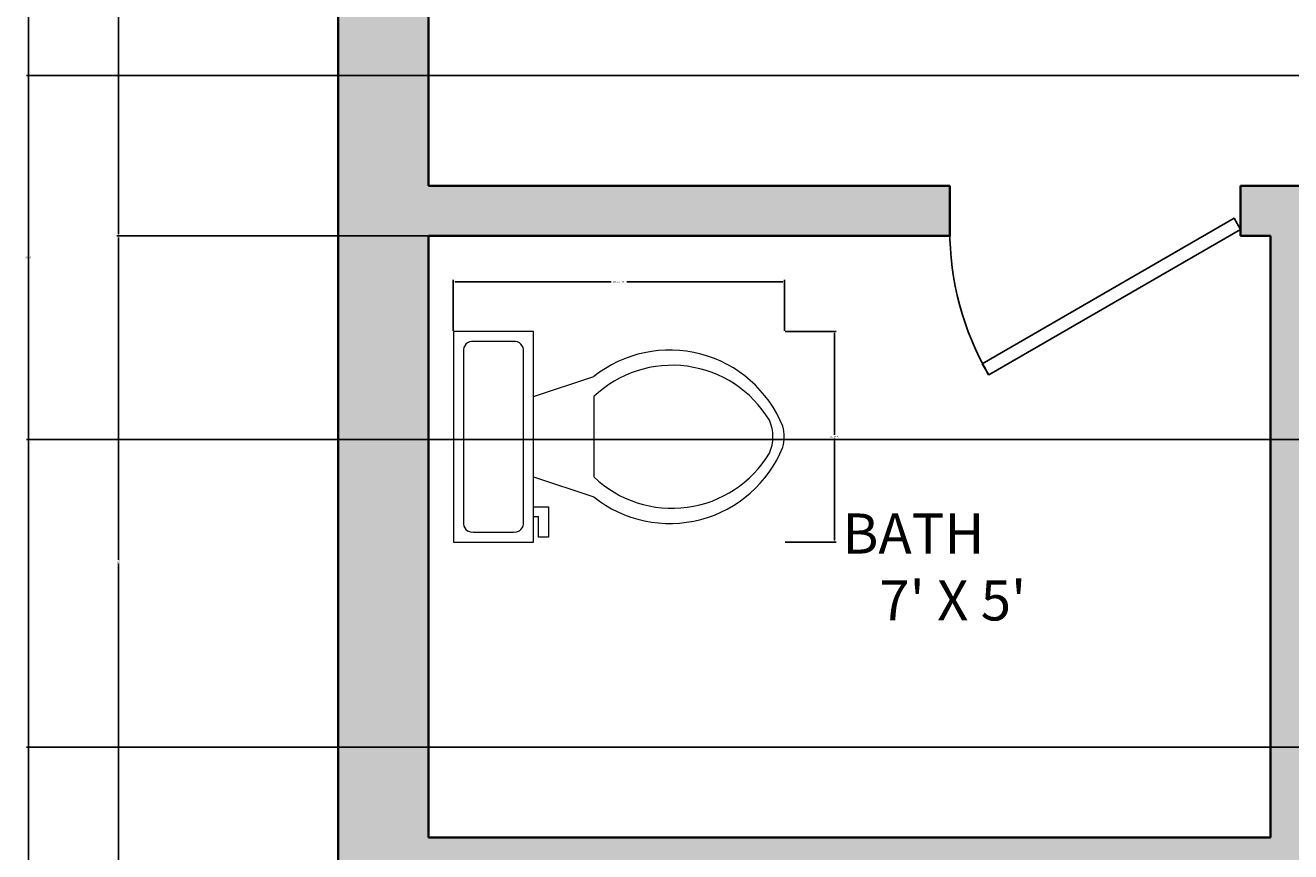
# Model space of a CAD drawing. Units: inches. Extents: x -30 to 437, y -29 to 647.
# Tile 3 of 15: x -30 to 97, y 172 to 255. Entities that reach past the tile are written whole.
import ezdxf

# ---------------------------------------------------------------- set-up
doc = ezdxf.new("R2010")
doc.units = ezdxf.units.IN
doc.header["$MEASUREMENT"] = 0
for name, color, linetype, lineweight in [('A-ANNO-DIMS', 2, 'Continuous', 18), ('A-AREA-IDEN', 7, 'Continuous', 18), ('A-WALL', 7, 'Continuous', 35), ('bathroom', 90, 'Continuous', 18), ('doors', 40, 'Continuous', 25)]:
    doc.layers.add(name, color=color, linetype=linetype, lineweight=lineweight)
doc.layers.add('A-WALL-PATT', color=251, linetype='Continuous', lineweight=13, true_color=0x636466)
doc.styles.get("Standard").update_dxf_attribs({"font": 'arial.ttf'})
doc.dimstyles.get("Standard").update_dxf_attribs({"dimtxt": 0.18, "dimasz": 0.18, "dimexe": 0.18, "dimexo": 0.0625, "dimgap": 0.09, "dimtad": 0, "dimtih": 1, "dimtoh": 1, "dimdec": 4, "dimzin": 0, "dimdsep": 46, "dimtxsty": 'Standard', "dimcen": 0.09, "dimadec": 0, "dimazin": 0, "dimtfac": 1, "dimtdec": 4, "dimtofl": 0, "dimtmove": 0, "dimatfit": 3, "dimfxl": 1, "dimtolj": 1, "dimtzin": 0, "dimarcsym": 0})

# ---------------------------------------------------------------- blocks, each defined once
blk = doc.blocks.new('Toilet - top')
for p, q in [((9.5, -6), (9.5, -2)), ((-10, -8.5), (-8, -8.5)), ((-10, -9.5), (-10, -8.5)), ((-8, -8.5), (-8, -8)), ((-7, -8), (-7, -9.5)), ((-4, -8), (-6, -14)), ((4, -8), (6, -14)), ((-7, -9.5), (-10, -9.5)), ((4, -14), (-4, -14))]:
    blk.add_line(p, q)
blk.add_lwpolyline([(10.5, -8), (10.5, 0), (-10.5, 0), (-10.5, -8)], close=True)
for points in [[(8.5, -1), (-8.5, -1)], [(-9.5, -2), (-9.5, -6)], [(-8.5, -7), (8.5, -7)]]:
    blk.add_lwpolyline(points)
for centre, radius, start, end in [((-8.62, -1.88), 0.884, 81.8699, 188.1301), ((8.62, -1.88), 0.884, 351.8699, 98.1301), ((-8.62, -6.12), 0.884, 171.8699, 278.1301), ((8.62, -6.12), 0.884, 261.8699, 8.1301), ((3.52, -21.58), 12.17, 141.4691, 247.9714), ((4.2, -21.82), 11.33, 136.3677, 238.9468), ((-3.52, -21.58), 12.17, 292.0284, 38.5307), ((-4.2, -21.82), 11.33, 301.053, 43.6321), ((0, -27.88), 4, 245.7318, 294.2682), ((0, -29), 4, 254.8605, 285.1395)]:
    blk.add_arc(centre, radius, start, end)
blk = doc.blocks.new('*U6')
for p, q in [((0, 0), (0, -6)), ((40, 0), (40, -6))]:
    blk.add_line(p, q)
blk.add_lwpolyline([(0, 0), (34.64, 20), (35.52, 18.48), (0.87, -1.52)], close=True)
blk.add_arc((0, 0), 40, 0, 30)
blk = doc.blocks.new('*D13')
at = {"layer": 'A-ANNO-DIMS', "color": 0, "lineweight": -2, "transparency": 16777216}
for p, q in [((13.16, 224.07), (13.16, 229.15)), ((13.34, 228.97), (28.91, 228.97)), ((46.03, 228.97), (30.46, 228.97)), ((46.21, 224.07), (46.21, 229.15))]:
    blk.add_line(p, q, dxfattribs=at)
at = {"layer": 'A-ANNO-DIMS', "color": 0, "transparency": 16777216}
for points in [[(13.34, 229), (13.34, 228.94), (13.16, 228.97)], [(46.03, 229), (46.03, 228.94), (46.21, 228.97)]]:
    blk.add_solid(points, dxfattribs=at)
at = {"layer": 'Defpoints', "color": 0, "transparency": 16777216}
for p in [(13.16, 228.97), (13.16, 224.01), (46.21, 224.01)]:
    blk.add_point(p, dxfattribs=at)
at = {"layer": 'A-ANNO-DIMS', "color": 0, "transparency": 16777216, "insert": (29.69, 228.97), "char_height": 0.18, "attachment_point": 5}
blk.add_mtext('\\A1;WC 33 TYP.', dxfattribs=at)
blk = doc.blocks.new('*D14')
at = {"layer": 'A-ANNO-DIMS', "color": 0, "lineweight": -2, "transparency": 16777216}
for p, q in [((46.27, 224.01), (51.35, 224.01)), ((51.17, 223.83), (51.17, 213.69)), ((51.17, 203.19), (51.17, 213.33)), ((46.27, 203.01), (51.35, 203.01))]:
    blk.add_line(p, q, dxfattribs=at)
at = {"layer": 'A-ANNO-DIMS', "color": 0, "transparency": 16777216}
for points in [[(51.14, 223.83), (51.2, 223.83), (51.17, 224.01)], [(51.14, 203.19), (51.2, 203.19), (51.17, 203.01)]]:
    blk.add_solid(points, dxfattribs=at)
at = {"layer": 'Defpoints', "color": 0, "transparency": 16777216}
for p in [(46.21, 224.01), (51.17, 224.01), (46.21, 203.01)]:
    blk.add_point(p, dxfattribs=at)
at = {"layer": 'A-ANNO-DIMS', "color": 0, "transparency": 16777216, "insert": (51.17, 213.51), "char_height": 0.18, "attachment_point": 5}
blk.add_mtext('\\A1;21 TYP.', dxfattribs=at)
blk = doc.blocks.new('*D26')
at = {"layer": 'A-ANNO-DIMS', "color": 0, "lineweight": -2, "transparency": 16777216}
for p, q in [((1.61, 615.55), (-29.41, 615.55)), ((-29.23, 615.37), (-29.23, 308.98)), ((-29.23, 2.23), (-29.23, 308.62)), ((1.61, 2.05), (-29.41, 2.05))]:
    blk.add_line(p, q, dxfattribs=at)
at = {"layer": 'A-ANNO-DIMS', "color": 0, "transparency": 16777216}
for points in [[(-29.26, 615.37), (-29.2, 615.37), (-29.23, 615.55)], [(-29.26, 2.23), (-29.2, 2.23), (-29.23, 2.05)]]:
    blk.add_solid(points, dxfattribs=at)
at = {"layer": 'Defpoints', "color": 0, "transparency": 16777216}
for p in [(-29.23, 615.55), (1.67, 615.55), (1.67, 2.05)]:
    blk.add_point(p, dxfattribs=at)
at = {"layer": 'A-ANNO-DIMS', "color": 0, "transparency": 16777216, "insert": (-29.23, 308.8), "char_height": 0.18, "attachment_point": 5}
blk.add_mtext('\\A1;613.5', dxfattribs=at)
blk = doc.blocks.new('*D31')
at = {"layer": 'A-ANNO-DIMS', "color": 0, "lineweight": -2, "transparency": 16777216}
for p, q in [((10.61, 233.55), (-20.41, 233.55)), ((-20.23, 233.37), (-20.23, 201.23)), ((-20.23, 168.73), (-20.23, 200.87)), ((10.61, 168.55), (-20.41, 168.55))]:
    blk.add_line(p, q, dxfattribs=at)
at = {"layer": 'A-ANNO-DIMS', "color": 0, "transparency": 16777216}
for points in [[(-20.26, 233.37), (-20.2, 233.37), (-20.23, 233.55)], [(-20.26, 168.73), (-20.2, 168.73), (-20.23, 168.55)]]:
    blk.add_solid(points, dxfattribs=at)
at = {"layer": 'Defpoints', "color": 0, "transparency": 16777216}
for p in [(-20.23, 233.55), (10.67, 233.55), (10.67, 168.55)]:
    blk.add_point(p, dxfattribs=at)
at = {"layer": 'A-ANNO-DIMS', "color": 0, "transparency": 16777216, "insert": (-20.23, 201.05), "char_height": 0.18, "attachment_point": 5}
blk.add_mtext('\\A1;65', dxfattribs=at)
blk = doc.blocks.new('*D32')
at = {"layer": 'A-ANNO-DIMS', "color": 0, "lineweight": -2, "transparency": 16777216}
for p, q in [((10.61, 386.55), (-20.41, 386.55)), ((-20.23, 386.37), (-20.23, 310.23)), ((-20.23, 233.73), (-20.23, 309.87)), ((10.61, 233.55), (-20.41, 233.55))]:
    blk.add_line(p, q, dxfattribs=at)
at = {"layer": 'A-ANNO-DIMS', "color": 0, "transparency": 16777216}
for points in [[(-20.26, 386.37), (-20.2, 386.37), (-20.23, 386.55)], [(-20.26, 233.73), (-20.2, 233.73), (-20.23, 233.55)]]:
    blk.add_solid(points, dxfattribs=at)
at = {"layer": 'Defpoints', "color": 0, "transparency": 16777216}
for p in [(-20.23, 386.55), (10.67, 386.55), (10.67, 233.55)]:
    blk.add_point(p, dxfattribs=at)
at = {"layer": 'A-ANNO-DIMS', "color": 0, "transparency": 16777216, "insert": (-20.23, 310.05), "char_height": 0.18, "attachment_point": 5}
blk.add_mtext('\\A1;153', dxfattribs=at)
blk = doc.blocks.new('*D52')
at = {"layer": 'A-ANNO-DIMS', "color": 0, "lineweight": -2, "transparency": 16777216}
for p, q in [((367.61, 182.55), (-29.41, 182.55)), ((-29.23, 182.37), (-29.23, 168.23)), ((-29.23, 153.73), (-29.23, 167.87)), ((396.61, 153.55), (-29.41, 153.55))]:
    blk.add_line(p, q, dxfattribs=at)
at = {"layer": 'A-ANNO-DIMS', "color": 0, "transparency": 16777216}
for points in [[(-29.26, 182.37), (-29.2, 182.37), (-29.23, 182.55)], [(-29.26, 153.73), (-29.2, 153.73), (-29.23, 153.55)]]:
    blk.add_solid(points, dxfattribs=at)
at = {"layer": 'Defpoints', "color": 0, "transparency": 16777216}
for p in [(367.67, 182.55), (-29.23, 153.55), (396.67, 153.55)]:
    blk.add_point(p, dxfattribs=at)
at = {"layer": 'A-ANNO-DIMS', "color": 0, "transparency": 16777216, "insert": (-29.23, 168.05), "char_height": 0.18, "attachment_point": 5}
blk.add_mtext('\\A1;29', dxfattribs=at)
blk = doc.blocks.new('*D55')
at = {"layer": 'A-ANNO-DIMS', "color": 0, "lineweight": -2, "transparency": 16777216}
for p, q in [((367.61, 249.55), (-29.41, 249.55)), ((-29.23, 249.37), (-29.23, 231.57)), ((-29.23, 213.42), (-29.23, 231.21)), ((369.54, 213.24), (-29.41, 213.24))]:
    blk.add_line(p, q, dxfattribs=at)
at = {"layer": 'A-ANNO-DIMS', "color": 0, "transparency": 16777216}
for points in [[(-29.26, 249.37), (-29.2, 249.37), (-29.23, 249.55)], [(-29.26, 213.42), (-29.2, 213.42), (-29.23, 213.24)]]:
    blk.add_solid(points, dxfattribs=at)
at = {"layer": 'Defpoints', "color": 0, "transparency": 16777216}
for p in [(-29.23, 249.55), (367.67, 249.55), (369.61, 213.24)]:
    blk.add_point(p, dxfattribs=at)
at = {"layer": 'A-ANNO-DIMS', "color": 0, "transparency": 16777216, "insert": (-29.23, 231.39), "char_height": 0.18, "attachment_point": 5}
blk.add_mtext('\\A1;36.31', dxfattribs=at)

msp = doc.modelspace()

# ---------------------------------------------------------------- hatches: boundary and pattern name
at = {"layer": 'A-WALL-PATT'}
h = msp.add_hatch(color=256, dxfattribs=at)
h.dxf.hatch_style = 1
h.paths.add_polyline_path([(393.6054, 183.2352), (369.6054, 183.2352), (369.6054, 213.2352), (393.6054, 213.2352), (393.6054, 207.2352), (394.6054, 207.2352), (394.6054, 211.2352), (395.6054, 211.2352), (395.6054, 185.2352), (394.6054, 185.2352), (394.6054, 189.2352), (393.6054, 189.2352)], flags=0)
h.paths.add_polyline_path([(384.6054, 189.2352, -1), (390.6054, 189.2352, -1)], flags=0)
h.paths.add_polyline_path([(385.6054, 189.2352, -1), (389.6054, 189.2352, -1)], flags=0)
h.paths.add_polyline_path([(374.6054, 189.2352, -1), (382.6054, 189.2352, -1)], flags=0)
h.paths.add_polyline_path([(386.6054, 189.2352, -1), (388.6054, 189.2352, -1)], flags=0)
h.paths.add_polyline_path([(375.6054, 189.2352, -1), (381.6054, 189.2352, -1)], flags=0)
h.paths.add_polyline_path([(376.6054, 189.2352, -1), (380.6054, 189.2352, -1)], flags=0)
h.paths.add_polyline_path([(377.6054, 189.2352, -1), (379.6054, 189.2352, -1)], flags=0)
h.paths.add_polyline_path([(390.6054, 195.2352), (374.6054, 195.2352), (374.6054, 201.2352), (390.6054, 201.2352)], flags=0)
h.paths.add_polyline_path([(389.6054, 196.2352), (375.6054, 196.2352), (375.6054, 200.2352), (389.6054, 200.2352)], flags=0)
h.paths.add_polyline_path([(383.6054, 207.2352, -1), (391.6054, 207.2352, -1)], flags=0)
h.paths.add_polyline_path([(384.6054, 207.2352, -1), (390.6054, 207.2352, -1)], flags=0)
h.paths.add_polyline_path([(385.6054, 207.2352, -1), (389.6054, 207.2352, -1)], flags=0)
h.paths.add_polyline_path([(386.6054, 207.2352, -1), (388.6054, 207.2352, -1)], flags=0)
h.paths.add_polyline_path([(375.6054, 207.2352, -1), (381.6054, 207.2352, -1)], flags=0)
h.paths.add_polyline_path([(376.6054, 207.2352, -1), (380.6054, 207.2352, -1)], flags=0)
h.paths.add_polyline_path([(377.6054, 207.2352, -1), (379.6054, 207.2352, -1)], flags=0)
h.paths.add_polyline_path([(305.5437, 160.3663, -0.41421356), (304.0437, 158.8663), (271.0437, 158.8663, -0.41421356), (269.5437, 160.3663), (269.5437, 178.3663, -0.41421356), (271.0437, 179.8663), (304.0437, 179.8663, -0.41421356), (305.5437, 178.3663)], flags=0)
h.paths.add_polyline_path([(304.0437, 165.3663, -0.41421356), (303.0437, 164.3663), (289.2937, 164.3663, -0.41421356), (288.2937, 165.3663), (288.2937, 177.3663, -0.41421356), (289.2937, 178.3663), (303.0437, 178.3663, -0.41421356), (304.0437, 177.3663)], flags=0)
h.paths.add_polyline_path([(296.5437, 171.3663, -1), (295.5437, 171.3663, -1)], flags=0)
h.paths.add_polyline_path([(286.7937, 165.3663, -0.41421356), (285.7937, 164.3663), (272.0437, 164.3663, -0.41421356), (271.0437, 165.3663), (271.0437, 177.3663, -0.41421356), (272.0437, 178.3663), (285.7937, 178.3663, -0.41421356), (286.7937, 177.3663)], flags=0)
h.paths.add_polyline_path([(279.5437, 171.3663, -1), (278.5437, 171.3663, -1)], flags=0)
h.paths.add_polyline_path([(360.6737, 290.5474), (360.6737, 300.5474), (396.6737, 300.5474), (396.6737, 290.5474)], flags=0)
h.paths.add_polyline_path([(259.6737, 124.5474), (259.6737, 114.5474), (171.6737, 114.5474), (171.6737, 124.5474)], flags=0)
h.paths.add_polyline_path([(288.0737, 215.3705), (286.7097, 214.583), (268.7097, 245.7599), (270.0737, 246.5474)], flags=0)
h.paths.add_polyline_path([(259.6737, 168.5474), (256.6737, 168.5474), (256.6737, 173.5474), (256.6737, 179.0224), (255.8753, 177.6395), (224.2956, 195.872, 0.12053744), (220.1737, 179.0224, 0.12053744), (216.0518, 195.872), (184.4721, 177.6395), (183.6737, 179.0224), (215.2836, 197.2724), (216.0821, 195.8895), (216.0518, 195.872, -0.12053744), (220.1737, 179.0224, -0.12053744), (224.2956, 195.872), (224.2653, 195.8895), (225.0638, 197.2724), (256.6737, 179.0224), (256.6737, 173.5474), (259.6737, 173.5474)], flags=0)
h.paths.add_polyline_path([(386.7943, 325.4601), (372.6871, 325.4601), (372.6871, 339.5673), (386.7943, 339.5673)], flags=0)
h.paths.add_polyline_path([(359.5875, 343.7429), (357.7905, 343.7429), (357.7905, 327.9179), (359.3933, 327.9179, 0.41420885), (361.5302, 330.0549), (361.5302, 341.8434, 0.41436161)], flags=0)
h.paths.add_polyline_path([(341.7887, 323.1235, -0.11921667), (340.7839, 323.1235)], flags=0)
h.paths.add_polyline_path([(379.6332, 328.8632), (379.6332, 332.2699), (376.0992, 332.2699, 0.39427733)], flags=0)
h.paths.add_polyline_path([(375.5299, 332.459, -1), (383.8511, 332.459, -1)], flags=0)
h.paths.add_polyline_path([(388.9363, 344.7425), (372.5309, 344.7425, -0.41421356), (370.394, 346.8794), (370.394, 347.5594, -0.39085173), (372.3472, 349.7005, -0.43951011), (370.394, 351.4933), (370.394, 365.1894, -0.40305452), (372.2191, 367.1298, -0.41839453), (370.394, 368.9291), (370.394, 382.6251, -0.40885826), (372.2519, 384.5722, -0.42377324), (370.394, 386.3707), (370.394, 400.0667, -0.38660687), (372.1327, 402.0094), (372.531, 402.0094, -0.41421834), (370.394, 404.1464), (370.394, 404.7778, -0.41420891), (372.5309, 406.9147), (388.9363, 406.9147, -0.41421821), (391.0733, 404.7778), (391.0733, 346.8794, -0.41421356)], flags=0)
edge = h.paths.add_edge_path(flags=0)
edge.add_spline(control_points=[(349.3585, 363.204), (349.0859, 363.204), (348.8133, 363.2227), (348.2712, 363.2973), (348.0016, 363.3531), (347.3533, 363.5328), (346.9776, 363.6755), (346.2445, 364.0308), (345.887, 364.2432), (345.1953, 364.7329), (344.8611, 365.0101), (344.2197, 365.6237), (343.9125, 365.9603), (343.211, 366.8336), (342.8313, 367.3965), (342.1401, 368.6117), (341.8286, 369.2641), (341.2807, 370.64), (341.0443, 371.3636), (340.6522, 372.8619), (340.4964, 373.6367), (340.2695, 375.2158), (340.1983, 376.0203), (340.142, 377.6365), (340.157, 378.4483), (340.2729, 380.0567), (340.3738, 380.8533), (340.6589, 382.4093), (340.8432, 383.1686), (341.2906, 384.629), (341.5538, 385.3301), (342.1531, 386.6544), (342.4891, 387.2776), (343.2266, 388.4288), (343.6281, 388.9567), (344.4879, 389.9012), (344.9463, 390.3178), (345.7981, 390.9428), (346.182, 391.1771), (346.9712, 391.5648), (347.3766, 391.7182), (348.2004, 391.9387), (348.6189, 392.0058), (349.4588, 392.0508), (349.8801, 392.0288), (350.7146, 391.8966), (351.1278, 391.7865), (351.9366, 391.4822), (352.3323, 391.2882), (353.0989, 390.8223), (353.4699, 390.5504), (354.1819, 389.9355), (354.5229, 389.5924), (355.1706, 388.8418), (355.4772, 388.4343), (356.1315, 387.4422), (356.4671, 386.8397), (357.0692, 385.5581), (357.3356, 384.879), (357.7933, 383.4624), (357.9846, 382.725), (358.2875, 381.2112), (358.3992, 380.4349), (358.5404, 378.8643), (358.5699, 378.0699), (358.546, 376.4841), (358.4926, 375.6928), (358.3042, 374.1343), (358.1692, 373.3672), (357.8207, 371.8774), (357.6072, 371.1549), (357.1067, 369.7735), (356.8196, 369.1148), (356.1782, 367.8787), (355.8238, 367.3013), (355.0551, 366.244), (354.6408, 365.7641), (353.7607, 364.9161), (353.2948, 364.5481), (352.445, 364.0149), (352.0701, 363.822), (351.3034, 363.5117), (350.9116, 363.3943), (350.1325, 363.2418), (349.7455, 363.204), (349.3585, 363.204)], knot_values=[3.14159265, 3.14159265, 3.14159265, 3.14159265, 3.22691715, 3.22691715, 3.31224165, 3.31224165, 3.43426671, 3.43426671, 3.55629177, 3.55629177, 3.67831683, 3.67831683, 3.8003419, 3.8003419, 3.97157384, 3.97157384, 4.14280577, 4.14280577, 4.31403771, 4.31403771, 4.48526965, 4.48526965, 4.65650159, 4.65650159, 4.82773353, 4.82773353, 4.99896547, 4.99896547, 5.1701974, 5.1701974, 5.34142934, 5.34142934, 5.51266128, 5.51266128, 5.68389322, 5.68389322, 5.85512516, 5.85512516, 5.98669107, 5.98669107, 6.11825699, 6.11825699, 6.24982291, 6.24982291, 6.38138882, 6.38138882, 6.51295474, 6.51295474, 6.64452065, 6.64452065, 6.77608657, 6.77608657, 6.90765249, 6.90765249, 7.0392184, 7.0392184, 7.20701563, 7.20701563, 7.37481286, 7.37481286, 7.54261009, 7.54261009, 7.71040732, 7.71040732, 7.87820455, 7.87820455, 8.04600178, 8.04600178, 8.21379901, 8.21379901, 8.38159624, 8.38159624, 8.54939347, 8.54939347, 8.7171907, 8.7171907, 8.88498794, 8.88498794, 9.05278517, 9.05278517, 9.17820699, 9.17820699, 9.30362881, 9.30362881, 9.42477796, 9.42477796, 9.42477796, 9.42477796], degree=3, periodic=0)
edge.add_line((341.1696, 384.3006), (341.2012, 384.2808))
edge = h.paths.add_edge_path(flags=0)
edge.add_line((344.3353, 388.7801), (344.317, 388.7915))
edge.add_ellipse((349.3585, 377.6204), major_axis=(0, -13.7895), ratio=0.62186025, start_angle=-244.867444, end_angle=-124.769923)
h.paths.add_polyline_path([(163.6737, 163.1474), (132.4968, 145.1474), (131.7093, 146.5114), (162.8862, 164.5114)], flags=0)
h.paths.add_polyline_path([(366.4355, 409.0896, -0.41423669), (364.2985, 406.9525, -0.4913499), (361.5302, 408.8973), (361.5302, 420.6405, 0.41421356), (359.3932, 422.7775), (357.7905, 422.7775), (357.7905, 406.9525), (359.6317, 406.9525, 0.42741026), (361.5332, 408.9757, 0.39869469), (363.6672, 406.9525, 0.51958103), (366.4355, 409.0895)], flags=0)
h.paths.add_polyline_path([(386.7943, 410.9671), (372.6871, 410.9671), (372.6871, 425.0742), (386.7943, 425.0742)], flags=0)
h.paths.add_polyline_path([(379.6332, 414.3701), (379.6332, 417.7768), (376.0992, 417.7768, 0.39427733)], flags=0)
h.paths.add_polyline_path([(375.5299, 417.966, -1), (383.8511, 417.966, -1)], flags=0)
h.paths.add_polyline_path([(150.0377, 351.583), (148.6737, 352.3705), (166.6737, 383.5474), (168.0377, 382.7599)], flags=0)
h.paths.add_polyline_path([(91.6737, 234.1974), (66.559, 219.6974), (65.9246, 220.7962), (91.0393, 235.2962)], flags=0)
h.paths.add_polyline_path([(255.4612, 443.5834), (254.6737, 444.9474), (285.8506, 462.9474), (286.6381, 461.5834)], flags=0)
h.paths.add_polyline_path([(176.2737, 394.5474), (158.2737, 425.7243), (159.6377, 426.5118), (177.6377, 395.3349)], flags=0)
h.paths.add_polyline_path([(243.6737, 439.5474), (243.0393, 438.4486), (217.9246, 452.9486), (218.559, 454.0474)], flags=0)
h.paths.add_polyline_path([(38.1264, 269.8429), (40.2408, 269.8429), (40.2408, 270.3508), (38.1264, 270.3508)], flags=0)
h.paths.add_polyline_path([(75.7157, 289.9439), (40.2408, 289.9439), (38.1264, 289.6524), (40.2408, 289.6524)], flags=0)
h.paths.add_polyline_path([(75.7157, 270.0846), (77.6447, 270.0846), (77.6697, 270.1626), (75.7175, 270.1626)], flags=0)
h.paths.add_polyline_path([(80.5373, 293.3002), (33.0467, 293.3002), (13.5054, 293.3002), (13.5054, 351.9244), (29.7898, 351.9244), (80.5373, 351.9244)], flags=0)
h.paths.add_polyline_path([(46.0261, 212.466, -0.50131678), (27.1651, 207.5106), (21.165, 209.5107), (21.165, 206.5107), (22.665, 206.5107), (22.665, 203.5107), (21.165, 203.5107), (21.165, 203.0107), (13.165, 203.0107), (13.165, 224.0107), (21.165, 224.0107), (21.165, 217.5107), (27.1649, 219.5106, -0.50132349), (46.0261, 214.5554, -0.13289091)], flags=0)
h.paths.add_polyline_path([(44.688, 211.8666, -0.48007965), (27.165, 209.5107), (27.165, 217.5107, -0.4800795), (44.688, 215.1547, -0.21500378)], flags=0)
h.paths.add_polyline_path([(19.415, 204.0107), (15.165, 204.0107, -0.41421356), (14.165, 204.7607), (14.165, 222.0107, -0.41421356), (14.915, 223.0107), (19.165, 223.0107, -0.41421356), (20.165, 222.2607), (20.165, 205.0107, -0.41421356)], flags=0)
h.paths.add_polyline_path([(32.7608, 269.0719), (31.8439, 269.0719), (31.8439, 268.6134), (13.5054, 268.6134), (13.5054, 291.5366), (31.8439, 291.5366), (32.7608, 291.0781), (32.7608, 280.9919, -1), (32.7608, 279.1581)], flags=0)
h.paths.add_polyline_path([(40.2408, 360.1436), (38.1264, 360.1436), (38.1264, 359.6357), (40.2408, 359.6357)], flags=0)
h.paths.add_polyline_path([(75.7157, 355.2807), (40.2408, 355.2807), (38.1264, 355.5722), (40.2408, 355.5722), (40.2408, 355.2807), (75.7157, 355.2807), (75.7157, 375.5982), (40.2408, 375.5982), (38.1264, 375.3817), (40.2408, 375.3817), (40.2408, 375.5982), (75.7157, 375.5982), (77.9733, 375.062), (75.7175, 375.062), (75.7175, 374.554)], flags=0)
h.paths.add_polyline_path([(42.8174, 299.814, 0.13867074), (34.1602, 294.603), (14.8081, 294.603), (14.8081, 350.6216), (29.8539, 350.6216, 0.09822056)], flags=0)
h.paths.add_polyline_path([(15.8636, 276.7781, -0.30640166), (20.3757, 283.4499), (20.3483, 290.6726), (31.4014, 290.7146), (31.4309, 282.9124), (26.8287, 282.895, -0.26006276), (30.241, 276.7781, -1)], flags=0)
h.paths.add_polyline_path([(26.1332, 276.7781), (23.0523, 273.6972), (19.9714, 276.7781), (23.0523, 279.8589), (23.0523, 283.9209), (21.3493, 283.9145), (20.7006, 283.5219), (20.6907, 286.1226), (23.2914, 286.1325), (25.8936, 285.7522), (27.1939, 285.7572), (28.4928, 286.1522), (31.0935, 286.1621), (31.0918, 286.6172), (25.6303, 286.5965), (25.616, 290.3675), (31.0775, 290.3882), (31.0918, 286.6172), (31.1034, 283.5614), (28.5027, 283.5515), (25.9005, 283.9317), (23.0523, 283.9209), (23.0523, 279.8589)], flags=0)
h.paths.add_polyline_path([(24.0793, 276.7781, -1), (22.0253, 276.7781, -1)], flags=0)
h.paths.add_polyline_path([(35.7687, 302.2895, -0.41421356), (35.2283, 301.2726), (22.2164, 297.2909, -0.41421356), (21.1995, 297.8313), (15.7317, 315.6996, -0.41421356), (16.2721, 316.7165), (18.8554, 317.507), (15.3721, 328.8904, -0.41421356), (15.9125, 329.9073), (28.9244, 333.889, -0.41421356), (29.9414, 333.3486), (35.4091, 315.4802, -0.41421356), (34.8687, 314.4633), (32.2854, 313.6728)], flags=0)
h.paths.add_polyline_path([(361.3728, 532.6207), (302.7487, 532.6207), (302.7487, 580.1113), (302.7487, 599.6527), (361.3728, 599.6527), (361.3728, 583.3682)], flags=0)
h.paths.add_polyline_path([(370.1, 575.0316), (370.1, 572.9172), (370.6079, 572.9172), (370.6079, 575.0316)], flags=0)
h.paths.add_polyline_path([(385.0466, 537.4423), (385.0466, 572.9172), (384.8302, 575.0316), (384.8302, 572.9172)], flags=0)
h.paths.add_polyline_path([(384.5104, 535.3262), (384.5104, 537.4406), (384.0025, 537.4406), (364.7291, 537.4423), (364.7291, 572.9172), (365.0206, 575.0316), (365.0206, 572.9172), (364.7291, 572.9172), (364.7291, 537.4423), (384.5884, 537.4423), (384.5884, 535.5133)], flags=0)
h.paths.add_polyline_path([(384.5884, 535.5133), (383.4945, 535.164), (383.4945, 537.4406), (382.9866, 535.3262), (382.9866, 537.4406), (383.4945, 535.3262), (383.4945, 537.4406), (384.5884, 537.4406)], flags=0)
h.paths.add_polyline_path([(23.874, 286.8174), (21.0132, 286.8065), (21.0004, 290.1875), (23.8612, 290.1983)], flags=0)
h.paths.add_polyline_path([(242.9824, 511.1667), (234.9824, 511.1667), (234.9824, 517.6667), (228.9825, 515.6667, -0.50132349), (210.1213, 520.622, -0.13289091), (210.1213, 522.7114, -0.50131678), (228.9823, 527.6667), (234.9824, 525.6667), (234.9824, 528.6667), (233.4824, 528.6667), (233.4824, 531.6667), (234.9824, 531.6667), (234.9824, 532.1667), (242.9824, 532.1667)], flags=0)
h.paths.add_polyline_path([(236.9824, 512.1667, -0.41421356), (235.9824, 512.9167), (235.9824, 530.1667, -0.41421356), (236.7324, 531.1667), (240.9824, 531.1667, -0.41421356), (241.9824, 530.4167), (241.9824, 513.1667, -0.41421356), (241.2324, 512.1667)], flags=0)
h.paths.add_polyline_path([(279.533, 537.4423), (279.533, 535.5133), (279.6111, 535.4884), (279.6111, 537.4406)], flags=0)
h.paths.add_polyline_path([(279.2913, 575.0316), (279.2913, 572.9172), (279.7992, 572.9172), (279.7992, 575.0316)], flags=0)
h.paths.add_polyline_path([(211.4594, 520.0227, -0.21500378), (211.4594, 523.3107, -0.48007965), (228.9824, 525.6667), (228.9824, 517.6667, -0.4800795)], flags=0)
h.paths.add_polyline_path([(32.7627, 354.1465), (31.8457, 354.1465), (31.8457, 353.688), (13.5054, 353.688), (13.5054, 376.6134), (31.8457, 376.6134), (32.7627, 376.1549), (32.7627, 366.0677, -1), (32.7627, 364.2337)], flags=0)
h.paths.add_polyline_path([(15.9446, 365.1507, -1), (30.3234, 365.1507, -1)], flags=0)
h.paths.add_polyline_path([(41.213, 428.467), (43.3274, 428.467), (43.3274, 428.9749), (41.213, 428.9749)], flags=0)
h.paths.add_polyline_path([(78.8022, 448.568), (43.3274, 448.568), (41.213, 448.2765), (43.3274, 448.2765)], flags=0)
h.paths.add_polyline_path([(78.8022, 428.7087), (80.7313, 428.7087), (80.7562, 428.7868), (78.804, 428.7868)], flags=0)
h.paths.add_polyline_path([(26.2152, 365.1507), (23.134, 362.0696), (20.0529, 365.1507), (23.134, 368.2319)], flags=0)
h.paths.add_polyline_path([(24.1611, 365.1507, -1), (22.107, 365.1507, -1)], flags=0)
h.paths.add_polyline_path([(309.2625, 570.3406, 0.13867074), (304.0514, 578.9978), (304.0514, 598.3499), (360.07, 598.3499), (360.07, 583.3041, 0.09822056)], flags=0)
h.paths.add_polyline_path([(246.6737, 552.5474), (129.6737, 552.5474), (129.6737, 606.5474), (246.6737, 606.5474)], flags=16)
h.paths.add_polyline_path([(373.6822, 580.3953), (363.595, 580.3953), (363.595, 581.3123), (363.1365, 581.3123), (363.1365, 599.6527), (386.0619, 599.6527), (386.0619, 581.3123), (385.6034, 580.3953), (375.5162, 580.3953, -1)], flags=0)
h.paths.add_polyline_path([(83.6239, 451.9244), (36.1333, 451.9244), (16.5919, 451.9244), (16.5919, 510.5485), (32.8764, 510.5485), (83.6239, 510.5485)], flags=0)
h.paths.add_polyline_path([(367.4098, 590.024, -1), (381.7886, 590.024, -1)], flags=0)
h.paths.add_polyline_path([(374.5992, 586.9428), (371.518, 590.024), (374.5992, 593.1052), (377.6803, 590.024)], flags=0)
h.paths.add_polyline_path([(373.5721, 590.024, -1), (375.6262, 590.024, -1)], flags=0)
h.paths.add_polyline_path([(324.9287, 577.7489, -0.41421356), (323.9118, 578.2893), (323.1212, 580.8726), (311.7379, 577.3893, -0.41421356), (310.721, 577.9297), (306.7393, 590.9416, -0.41421356), (307.2797, 591.9585), (325.1481, 597.4263, -0.41421356), (326.165, 596.8859), (326.9555, 594.3026), (338.3388, 597.7859, -0.41421356), (339.3557, 597.2455), (343.3374, 584.2336, -0.41421356), (342.797, 583.2167)], flags=0)
h.paths.add_polyline_path([(300.5265, 580.3972), (290.4404, 580.3972, -1), (288.6065, 580.3972), (278.5203, 580.3972), (278.5203, 581.3142), (278.0619, 581.3142), (278.0619, 599.6527), (300.985, 599.6527), (300.985, 581.3142)], flags=0)
h.paths.add_polyline_path([(300.163, 581.7567), (292.3609, 581.7271), (292.3434, 586.3294, -0.75567924), (279.0378, 590.1057, -0.82536731), (292.8983, 592.7823), (300.1211, 592.8097)], flags=0)
h.paths.add_polyline_path([(299.8367, 582.0805), (296.0656, 582.0662), (293.0098, 582.0546), (292.9999, 584.6553), (293.3802, 587.2575), (293.3694, 590.1057), (289.3074, 590.1057), (286.2265, 587.0248), (283.1456, 590.1057), (286.2265, 593.1866), (289.3074, 590.1057), (293.3694, 590.1057), (293.3629, 591.8088), (292.9703, 592.4575), (295.5711, 592.4673), (295.5809, 589.8666), (295.2007, 587.2644), (295.2056, 585.9641), (295.6006, 584.6652), (295.6105, 582.0645), (296.0656, 582.0662), (296.0449, 587.5277), (299.8159, 587.542)], flags=0)
h.paths.add_polyline_path([(285.1995, 590.1057, -1), (287.2535, 590.1057, -1)], flags=0)
h.paths.add_polyline_path([(299.6467, 589.2969), (296.2658, 589.284), (296.255, 592.1448), (299.6359, 592.1576)], flags=0)
h.paths.add_polyline_path([(35.8473, 427.696), (34.9304, 427.696), (34.9304, 427.2376), (16.5919, 427.2376), (16.5919, 450.1607), (34.9304, 450.1607), (35.8473, 449.7022), (35.8473, 439.6161, -1), (35.8473, 437.7822)], flags=0)
h.paths.add_polyline_path([(18.9502, 435.4022, -0.30640166), (23.4623, 442.074), (23.4349, 449.2968), (34.4879, 449.3387), (34.5175, 441.5366), (29.9152, 441.5191, -0.26006276), (33.3275, 435.4022, -1)], flags=0)
h.paths.add_polyline_path([(29.2197, 435.4022), (26.1389, 432.3213), (23.058, 435.4022), (26.1389, 438.4831), (26.1389, 442.5451), (24.4358, 442.5386), (23.7871, 442.1461), (23.7772, 444.7468), (26.378, 444.7566), (28.9801, 444.3764), (30.2805, 444.3813), (31.5794, 444.7764), (34.1801, 444.7862), (34.1784, 445.2413), (28.7169, 445.2206), (28.7026, 448.9917), (34.164, 449.0124), (34.1784, 445.2413), (34.1899, 442.1855), (31.5892, 442.1756), (28.987, 442.5559), (26.1389, 442.5451), (26.1389, 438.4831)], flags=0)
h.paths.add_polyline_path([(27.1658, 435.4022, -1), (25.1119, 435.4022, -1)], flags=0)
h.paths.add_polyline_path([(45.904, 458.4382, 0.13867074), (37.2467, 453.2271), (17.8947, 453.2271), (17.8947, 509.2457), (32.9405, 509.2457, 0.09822056)], flags=0)
h.paths.add_polyline_path([(26.9605, 445.4415), (24.0997, 445.4307), (24.0869, 448.8116), (26.9477, 448.8225)], flags=0)
h.paths.add_polyline_path([(38.3149, 459.8967), (25.3029, 455.915, -0.41421356), (24.286, 456.4554), (18.8183, 474.3238, -0.41421356), (19.3586, 475.3407), (21.942, 476.1312), (18.4587, 487.5145, -0.41421356), (18.999, 488.5314), (32.011, 492.5131, -0.41421356), (33.0279, 491.9727), (38.4957, 474.1044, -0.41421356), (37.9553, 473.0875), (35.3719, 472.297), (38.8553, 460.9136, -0.41421356)], flags=0)
h.paths.add_polyline_path([(43.3274, 518.7678), (41.213, 518.7678), (41.213, 518.2598), (43.3274, 518.2598)], flags=0)
h.paths.add_polyline_path([(78.8022, 513.9049), (43.3274, 513.9049), (41.213, 514.1964), (43.3274, 514.1964), (43.3274, 513.9049), (78.8022, 513.9049), (78.8022, 534.2223), (43.3274, 534.2223), (41.213, 534.0059), (43.3274, 534.0059), (43.3274, 534.2223), (78.8022, 534.2223), (81.0599, 533.6861), (78.804, 533.6861), (78.804, 533.1782)], flags=0)
h.paths.add_polyline_path([(121.6737, 556.8974), (121.0393, 555.7986), (95.9246, 570.2986), (96.559, 571.3974)], flags=0)
h.paths.add_polyline_path([(35.8493, 512.7707), (34.9322, 512.7707), (34.9322, 512.3122), (16.5919, 512.3122), (16.5919, 535.2376), (34.9322, 535.2376), (35.8493, 534.7791), (35.8493, 524.6919, -1), (35.8493, 522.8579)], flags=0)
h.paths.add_polyline_path([(19.0312, 523.7749, -1), (33.41, 523.7749, -1)], flags=0)
h.paths.add_polyline_path([(26.2206, 520.6937), (23.1394, 523.7749), (26.2206, 526.8561), (29.3018, 523.7749)], flags=0)
h.paths.add_polyline_path([(25.1935, 523.7749, -1), (27.2476, 523.7749, -1)], flags=0)
h.paths.add_polyline_path([(28.4381, 586.0173), (22.438, 588.0173), (22.438, 585.0173), (23.938, 585.0173), (23.938, 582.0173), (22.438, 582.0173), (22.438, 581.5173), (14.438, 581.5173), (14.438, 602.5173), (22.438, 602.5173), (22.438, 596.0173), (28.4379, 598.0173, -0.50132349), (47.2992, 593.062, -0.13289091), (47.2992, 590.9726, -0.50131678)], flags=0)
h.paths.add_polyline_path([(28.438, 588.0174), (28.438, 596.0173, -0.4800795), (45.961, 593.6614, -0.21500378), (45.961, 590.3733, -0.48007965)], flags=0)
h.paths.add_polyline_path([(20.688, 582.5173), (16.438, 582.5173, -0.41421356), (15.438, 583.2673), (15.438, 600.5173, -0.41421356), (16.188, 601.5173), (20.438, 601.5173, -0.41421356), (21.438, 600.7673), (21.438, 583.5173, -0.41421356)], flags=0)
h.paths.add_polyline_path([(171.6737, 2.0474), (171.6737, 104.5474), (259.6737, 104.5474), (259.6737, 148.5474), (396.6737, 148.5474), (396.6737, 2.0474), (405.6737, 2.0474), (405.6737, 615.5474), (1.6737, 615.5474), (1.6737, 2.0474)])
h.paths.add_polyline_path([(171.6737, 104.5474), (259.6737, 104.5474), (259.6737, 210.5474), (264.6737, 210.5474), (264.6737, 153.5474), (396.6737, 153.5474), (396.6737, 249.5474), (264.6737, 249.5474), (264.6737, 246.5474), (259.6737, 246.5474), (259.6737, 254.5474), (396.6737, 254.5474), (396.6737, 434.5474), (290.6737, 434.5474), (290.6737, 439.5474), (396.6737, 439.5474), (396.6737, 606.5474), (251.6737, 606.5474), (251.6737, 439.5474), (254.6737, 439.5474), (254.6737, 434.5474), (243.6737, 434.5474), (243.6737, 439.5474), (246.6737, 439.5474), (246.6737, 547.5474), (186.6737, 547.5474), (186.6737, 439.5474), (214.6737, 439.5474), (214.6737, 434.5474), (186.6737, 434.5474), (186.6737, 430.5474), (181.6737, 430.5474), (181.6737, 547.5474), (121.6737, 547.5474), (121.6737, 552.5474), (124.6737, 552.5474), (124.6737, 606.5474), (10.6737, 606.5474), (10.6737, 552.5474), (92.6737, 552.5474), (92.6737, 547.5474), (10.6737, 547.5474), (10.6737, 391.5474), (181.6737, 391.5474), (181.6737, 394.5474), (186.6737, 394.5474), (186.6737, 386.5474), (171.6737, 386.5474), (171.6737, 383.5474), (166.6737, 383.5474), (166.6737, 386.5474), (10.6737, 386.5474), (10.6737, 238.5474), (62.6737, 238.5474), (62.6737, 233.5474), (10.6737, 233.5474), (10.6737, 173.5474), (94.6737, 173.5474), (94.6737, 233.5474), (91.6737, 233.5474), (91.6737, 238.5474), (166.6737, 238.5474), (166.6737, 347.5474), (171.6737, 347.5474), (171.6737, 233.5474), (99.6737, 233.5474), (99.6737, 173.5474), (127.6737, 173.5474), (127.6737, 168.5474), (10.6737, 168.5474), (10.6737, 11.0474), (166.6737, 11.0474), (166.6737, 168.5474), (163.6737, 168.5474), (163.6737, 173.5474), (183.6737, 173.5474), (183.6737, 168.5474), (171.6737, 168.5474)])

# ---------------------------------------------------------------- linework, layer by layer
at = {"layer": 'A-WALL'}
for p, q in [((10.6737, 238.5474), (10.6737, 386.5474)), ((10.6737, 238.5474), (62.6737, 238.5474)), ((62.6737, 233.5474), (62.6737, 238.5474)), ((91.6737, 238.5474), (166.6737, 238.5474)), ((94.6737, 238.5474), (91.6737, 238.5474)), ((91.6737, 238.5474), (91.6737, 233.5474)), ((10.6737, 233.5474), (62.6737, 233.5474)), ((10.6737, 173.5474), (10.6737, 233.5474)), ((91.6737, 233.5474), (94.6737, 233.5474)), ((94.6737, 173.5474), (94.6737, 233.5474)), ((10.6737, 173.5474), (94.6737, 173.5474))]:
    msp.add_line(p, q, dxfattribs=at)
msp.add_lwpolyline([(171.6737, 2.0474), (1.6737, 2.0474), (1.6737, 615.5474), (405.6737, 615.5474), (405.6737, 2.0474), (396.6737, 2.0474)], dxfattribs=at)

# ---------------------------------------------------------------- block references
at = {"layer": 'bathroom', "rotation": 90}
msp.add_blockref('Toilet - top', (13.165, 213.5107), dxfattribs=at)
at = {"layer": 'doors', "xscale": 0.725, "yscale": 0.725, "zscale": 0.725, "rotation": 180}
msp.add_blockref('*U6', (91.6737, 234.1974), dxfattribs=at)

# ---------------------------------------------------------------- texts
at = {"layer": 'A-AREA-IDEN', "insert": (50.7575, 205.8596), "char_height": 4, "attachment_point": 1}
msp.add_mtext_dynamic_manual_height_columns(" BATH\\P    7' X 5'", width=25.99481, gutter_width=1, heights=[0], dxfattribs=at)

# ---------------------------------------------------------------- dimensions: what is measured, and where the dimension line sits
at = {"layer": 'A-ANNO-DIMS'}
for base, p1, p2, override, picture, middle in [((-29.2263, 615.5474), (1.6737, 2.0474), (1.6737, 615.5474), {"dimdec": 1, "dimlfac": 1, "dimrnd": 0, "dimzin": 0, "dimdsep": 46, "dimlunit": 2}, '*D26', (-29.2263, 308.7974)), ((-20.2263, 386.5474), (10.6737, 233.5474), (10.6737, 386.5474), {"dimdec": 0, "dimlfac": 1, "dimrnd": 0, "dimzin": 0, "dimdsep": 46, "dimlunit": 2}, '*D32', (-20.2263, 310.0474)), ((-29.2263, 249.5474), (369.6054, 213.2352), (367.6737, 249.5474), {"dimdec": 2, "dimlfac": 1, "dimrnd": 0, "dimzin": 0, "dimdsep": 46, "dimlunit": 2}, '*D55', (-29.2263, 231.3913)), ((-20.2263, 233.5474), (10.6737, 168.5474), (10.6737, 233.5474), {"dimdec": 0, "dimlfac": 1, "dimrnd": 0, "dimzin": 0, "dimdsep": 46, "dimlunit": 2}, '*D31', (-20.2263, 201.0474)), ((-29.2263, 153.5474), (367.6737, 182.5474), (396.6737, 153.5474), {"dimdec": 0, "dimlfac": 1, "dimrnd": 0, "dimzin": 0, "dimdsep": 46, "dimlunit": 2}, '*D52', (-29.2263, 168.0474))]:
    dim = msp.add_linear_dim(base=base, p1=p1, p2=p2, angle=90, dimstyle='Standard', override=override, dxfattribs=at)
    dim.commit()
    dim.dimension.update_dxf_attribs({"geometry": picture, "text_midpoint": middle})
for base, p1, p2, angle, text, picture, middle in [((13.165, 228.9676), (46.2112, 224.0107), (13.165, 224.0107), 180, 'WC <> TYP.', '*D13', (29.6881, 228.9676)), ((51.1682, 224.0107), (46.2112, 203.0107), (46.2112, 224.0107), 90, '<> TYP.', '*D14', (51.1682, 213.5107))]:
    dim = msp.add_linear_dim(base=base, p1=p1, p2=p2, angle=angle, text=text, dimstyle='Standard', override={"dimdec": 0, "dimlfac": 1, "dimrnd": 0, "dimzin": 0, "dimdsep": 46, "dimlunit": 2}, dxfattribs=at)
    dim.commit()
    dim.dimension.update_dxf_attribs({"geometry": picture, "text_midpoint": middle})

doc.saveas('drawing.dxf')
